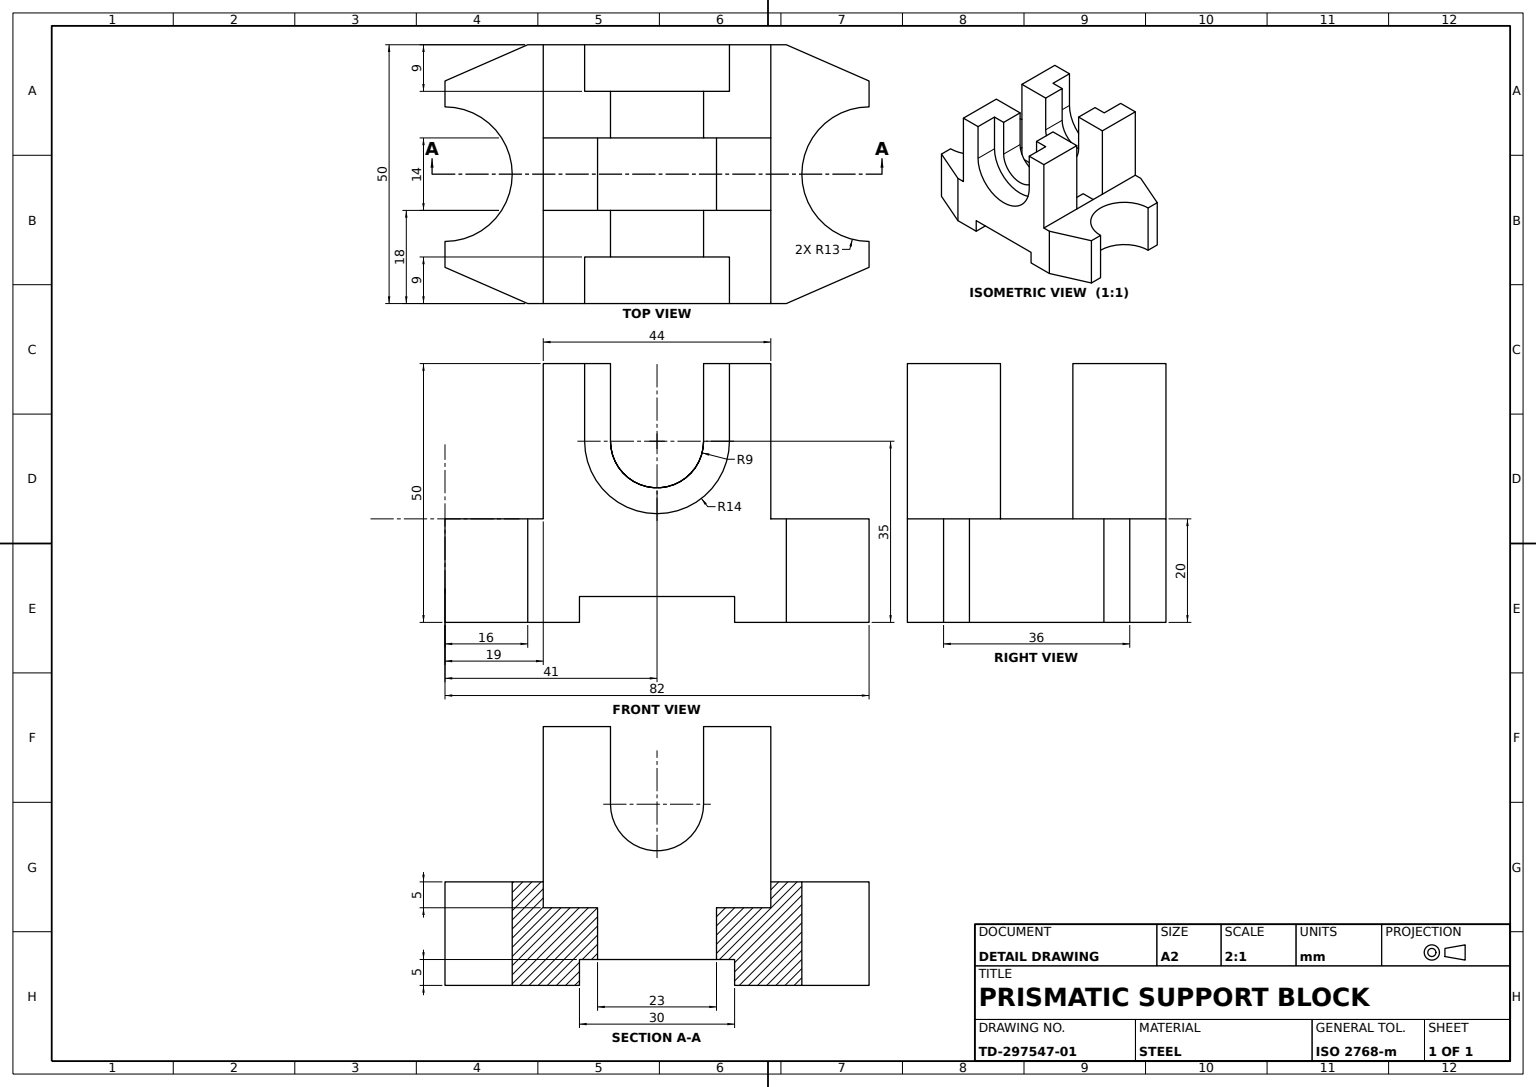
SolidWorks part; units mm, degrees
material "Plain Carbon Steel"
ref_plane "Front Plane" through (0, 0, 0) normal (0, 0, 1) x (1, 0, 0)
ref_plane "Top Plane" through (0, 0, 0) normal (0, 1, 0) x (1, 0, 0)
ref_plane "Right Plane" through (0, 0, 0) normal (1, 0, 0) x (0, 0, -1)
sketch "Base Block Profile" plane through (0, 0, 0) normal (0, 1, 0) x (1, 0, 0)
  line L0 (-25, 25) -> (25, 25)
  line L1 (25, 25) -> (41, 18)
  line L2 (41, 18) -> (41, 13)
  line L3 (41, -13) -> (41, -18)
  line L4 (41, -18) -> (25, -25)
  line L5 (25, -25) -> (-25, -25)
  line L6 (0, 0) -> (0, 6.6942) construction
  line L7 (0, 0) -> (5.7025, 0) construction
  line L8 (-41, 18) -> (-41, 13)
  line L9 (-25, 25) -> (-41, 18)
  line L10 (-41, -13) -> (-41, -18)
  line L11 (-41, -18) -> (-25, -25)
  arc A0 (41, 13) -> (41, -13) centre (41, 0) ccw
  arc A1 (-41, 13) -> (-41, -13) centre (-41, 0) cw
  dimension "D1" = 36
  dimension "D2" = 26
  dimension "D3" = 82
  dimension "D4" = 50
  dimension "D5" = 50
extrude "Base Block" add sketch "Base Block Profile" along normal blind 20
sketch "Uprights Profile" plane through (0, 0, 25) normal (0, 0, 1) x (1, 0, 0)
  line L0 (-22, 20) -> (-22, 50)
  line L1 (-25, 20) -> (25, 20) construction
  line L2 (-22, 50) -> (-9, 50)
  line L3 (-9, 50) -> (-9, 35)
  line L4 (9, 35) -> (9, 50)
  line L5 (9, 50) -> (22, 50)
  line L6 (22, 50) -> (22, 20)
  line L7 (22, 20) -> (-22, 20)
  arc A0 (-9, 35) -> (9, 35) centre (0, 35) ccw
  point P15 (0, 26)
  dimension "D2" = 9
  dimension "D4" = 6
  dimension "D1" = 44
  dimension "D3" = 50
extrude "Uprights" add sketch "Uprights Profile" against normal blind 18
sketch "Upright Notch Profile" plane through (0, 0, 25) normal (0, 0, 1) x (1, 0, 0)
  line L3 (-14, 50) -> (14, 50)
  line L5 (14, 50) -> (14, 35)
  line L6 (-14, 35) -> (-14, 50)
  line L7 (14, 50) -> (14, 35)
  line L8 (-14, 35) -> (-14, 50)
  arc A4 (-14, 35) -> (14, 35) centre (0, 35) ccw
  arc A5 (-14, 35) -> (14, 35) centre (0, 35) ccw
  dimension "D1" = 5
extrude "Upright Notch" cut sketch "Upright Notch Profile" against normal blind 9
mirror "Upright Notch Mirror" about plane through (0, 0, 0) normal (0, 0, 1) of "Upright Notch", "Uprights"
sketch "Underside Slot Profile" plane through (0, 0, 25) normal (0, 0, 1) x (1, 0, 0)
  line L0 (-25, 0) -> (25, 0) construction
  line L1 (-15, -5) -> (15, -5)
  line L2 (-15, -5) -> (-15, 5)
  line L3 (-15, 5) -> (15, 5)
  line L4 (15, -5) -> (15, 5)
  line L5 (-15, -5) -> (15, 5) construction
  line L6 (-15, 5) -> (15, -5) construction
  point P0 (0, 0)
  point P6 (15, 0)
  dimension "D1" = 30
  dimension "D2" = 5
extrude "Underside Slot" cut sketch "Underside Slot Profile" against normal through all
sketch "Saddle Cut Profile" plane through (0, 20, 0) normal (0, 1, 0) x (1, 0, 0)
  line L1 (-11.5, -7) -> (11.5, -7)
  line L2 (-11.5, -7) -> (-11.5, 7)
  line L3 (-11.5, 7) -> (11.5, 7)
  line L4 (11.5, -7) -> (11.5, 7)
  line L5 (-11.5, -7) -> (11.5, 7) construction
  line L6 (-11.5, 7) -> (11.5, -7) construction
  point P0 (0, 0)
  dimension "D1" = 14
  dimension "D2" = 23
extrude "Saddle Cut" cut sketch "Saddle Cut Profile" against normal through all
sketch "Upright Slot Profile" plane through (0, 20, 0) normal (0, 1, 0) x (1, 0, 0)
  line L1 (-22, 7) -> (22, 7)
  line L2 (-22, 7) -> (-22, -7)
  line L3 (-22, -7) -> (22, -7)
  line L4 (22, 7) -> (22, -7)
extrude "Upright Slot Cut" cut sketch "Upright Slot Profile" against normal blind 5
